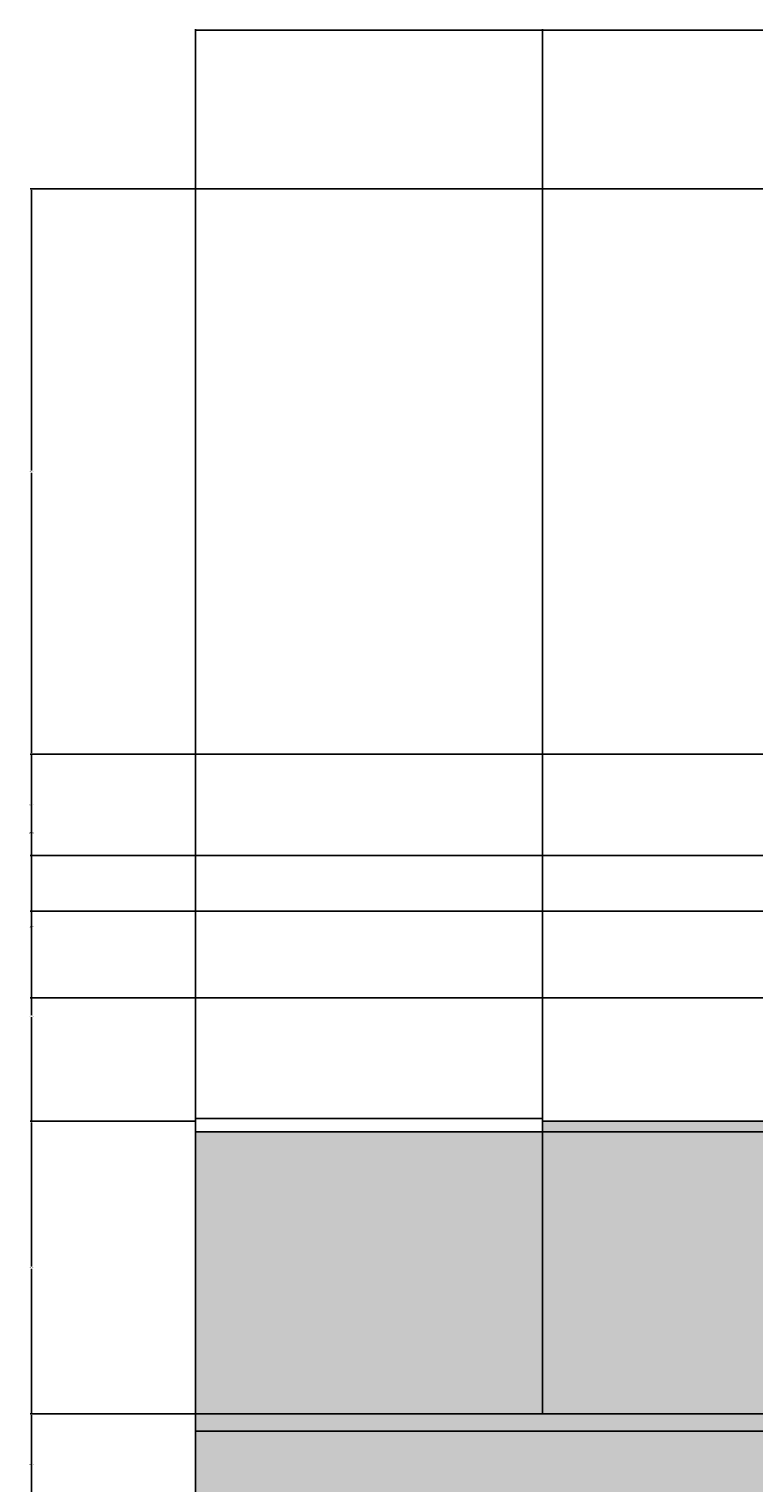
# Model space of a CAD drawing. Units: feet. Extents: x 2926 to 4178, y 965 to 1469.
# Tile 4 of 9: x 2926 to 3040, y 1241 to 1469. Entities that reach past the tile are written whole.
import ezdxf

# ---------------------------------------------------------------- set-up
doc = ezdxf.new("R2010")
doc.units = ezdxf.units.FT
for name, color, linetype, lineweight in [('A-ANNO-DIMS', 2, 'Continuous', 18), ('A-ELEV', 7, 'Continuous', 25), ('A-ELEV-PATT', 9, 'Continuous', 13)]:
    doc.layers.add(name, color=color, linetype=linetype, lineweight=lineweight)
doc.styles.get("Standard").update_dxf_attribs({"font": 'arial.ttf'})
doc.dimstyles.get("Standard").update_dxf_attribs({"dimtxt": 0.18, "dimasz": 0.18, "dimexe": 0.18, "dimexo": 0.0625, "dimgap": 0.09, "dimtad": 0, "dimtih": 1, "dimtoh": 1, "dimdec": 1, "dimzin": 0, "dimdsep": 46, "dimlunit": 3, "dimtxsty": 'Standard', "dimcen": 0.09, "dimadec": 0, "dimazin": 0, "dimtfac": 1, "dimtdec": 1, "dimtofl": 0, "dimtmove": 0, "dimatfit": 3, "dimfxl": 1, "dimtolj": 1, "dimtzin": 0, "dimarcsym": 0})

# ---------------------------------------------------------------- blocks, each defined once
blk = doc.blocks.new('*D10')
at = {"layer": 'A-ANNO-DIMS', "color": 0, "lineweight": -2, "transparency": 16777216}
for p, q in [((2952.4, 1298.4), (2952.4, 1468.62)), ((2952.58, 1468.44), (3195.09, 1468.44)), ((3438.39, 1468.44), (3195.88, 1468.44)), ((3438.57, 1443.71), (3438.57, 1468.62))]:
    blk.add_line(p, q, dxfattribs=at)
at = {"layer": 'A-ANNO-DIMS', "color": 0, "transparency": 16777216}
for points in [[(2952.58, 1468.47), (2952.58, 1468.41), (2952.4, 1468.44)], [(3438.39, 1468.47), (3438.39, 1468.41), (3438.57, 1468.44)]]:
    blk.add_solid(points, dxfattribs=at)
at = {"layer": 'Defpoints', "color": 0, "transparency": 16777216}
for p in [(3438.57, 1468.44), (3438.57, 1443.64), (2952.4, 1298.33)]:
    blk.add_point(p, dxfattribs=at)
at = {"layer": 'A-ANNO-DIMS', "color": 0, "transparency": 16777216, "insert": (3195.49, 1468.44), "char_height": 0.18, "attachment_point": 5}
blk.add_mtext('\\A1;486.2', dxfattribs=at)
blk = doc.blocks.new('*D17')
at = {"layer": 'A-ANNO-DIMS', "color": 0, "lineweight": -2, "transparency": 16777216}
for p, q in [((2952.34, 1252.14), (2926.57, 1252.14)), ((2926.75, 1251.96), (2926.75, 1235.86)), ((2926.75, 1219.4), (2926.75, 1235.5)), ((3198.58, 1219.22), (2926.57, 1219.22))]:
    blk.add_line(p, q, dxfattribs=at)
at = {"layer": 'A-ANNO-DIMS', "color": 0, "transparency": 16777216}
for points in [[(2926.72, 1251.96), (2926.78, 1251.96), (2926.75, 1252.14)], [(2926.72, 1219.4), (2926.78, 1219.4), (2926.75, 1219.22)]]:
    blk.add_solid(points, dxfattribs=at)
at = {"layer": 'Defpoints', "color": 0, "transparency": 16777216}
for p in [(2926.75, 1252.14), (2952.4, 1252.14), (3198.64, 1219.22)]:
    blk.add_point(p, dxfattribs=at)
at = {"layer": 'A-ANNO-DIMS', "color": 0, "transparency": 16777216, "insert": (2926.75, 1235.68), "char_height": 0.18, "attachment_point": 5}
blk.add_mtext('\\A1;32.92', dxfattribs=at)
blk = doc.blocks.new('*D18')
at = {"layer": 'A-ANNO-DIMS', "color": 0, "lineweight": -2, "transparency": 16777216}
for p, q in [((2952.34, 1297.9), (2926.57, 1297.9)), ((2926.75, 1297.72), (2926.75, 1275.2)), ((2926.75, 1252.32), (2926.75, 1274.84)), ((2952.34, 1252.14), (2926.57, 1252.14))]:
    blk.add_line(p, q, dxfattribs=at)
at = {"layer": 'A-ANNO-DIMS', "color": 0, "transparency": 16777216}
for points in [[(2926.72, 1297.72), (2926.78, 1297.72), (2926.75, 1297.9)], [(2926.72, 1252.32), (2926.78, 1252.32), (2926.75, 1252.14)]]:
    blk.add_solid(points, dxfattribs=at)
at = {"layer": 'Defpoints', "color": 0, "transparency": 16777216}
for p in [(2926.75, 1297.9), (2952.4, 1297.9), (2952.4, 1252.14)]:
    blk.add_point(p, dxfattribs=at)
at = {"layer": 'A-ANNO-DIMS', "color": 0, "transparency": 16777216, "insert": (2926.75, 1275.02), "char_height": 0.18, "attachment_point": 5}
blk.add_mtext('\\A1;45.76', dxfattribs=at)
blk = doc.blocks.new('*D19')
at = {"layer": 'A-ANNO-DIMS', "color": 0, "lineweight": -2, "transparency": 16777216}
for p, q in [((3335.85, 1330.74), (2926.57, 1330.74)), ((2926.75, 1330.56), (2926.75, 1314.5)), ((2926.75, 1298.08), (2926.75, 1314.14)), ((2952.34, 1297.9), (2926.57, 1297.9))]:
    blk.add_line(p, q, dxfattribs=at)
at = {"layer": 'A-ANNO-DIMS', "color": 0, "transparency": 16777216}
for points in [[(2926.72, 1330.56), (2926.78, 1330.56), (2926.75, 1330.74)], [(2926.72, 1298.08), (2926.78, 1298.08), (2926.75, 1297.9)]]:
    blk.add_solid(points, dxfattribs=at)
at = {"layer": 'Defpoints', "color": 0, "transparency": 16777216}
for p in [(2926.75, 1330.74), (3335.91, 1330.74), (2952.4, 1297.9)]:
    blk.add_point(p, dxfattribs=at)
at = {"layer": 'A-ANNO-DIMS', "color": 0, "transparency": 16777216, "insert": (2926.75, 1314.32), "char_height": 0.18, "attachment_point": 5}
blk.add_mtext('\\A1;32.85', dxfattribs=at)
blk = doc.blocks.new('*D20')
at = {"layer": 'A-ANNO-DIMS', "color": 0, "lineweight": -2, "transparency": 16777216}
for p, q in [((3042.86, 1355.28), (2926.57, 1355.28)), ((2926.75, 1355.1), (2926.75, 1343.19)), ((2926.75, 1330.92), (2926.75, 1342.83)), ((3335.85, 1330.74), (2926.57, 1330.74))]:
    blk.add_line(p, q, dxfattribs=at)
at = {"layer": 'A-ANNO-DIMS', "color": 0, "transparency": 16777216}
for points in [[(2926.72, 1355.1), (2926.78, 1355.1), (2926.75, 1355.28)], [(2926.72, 1330.92), (2926.78, 1330.92), (2926.75, 1330.74)]]:
    blk.add_solid(points, dxfattribs=at)
at = {"layer": 'Defpoints', "color": 0, "transparency": 16777216}
for p in [(2926.75, 1355.28), (3042.92, 1355.28), (3335.91, 1330.74)]:
    blk.add_point(p, dxfattribs=at)
at = {"layer": 'A-ANNO-DIMS', "color": 0, "transparency": 16777216, "insert": (2926.75, 1343.01), "char_height": 0.18, "attachment_point": 5}
blk.add_mtext('\\A1;24.533', dxfattribs=at)
blk = doc.blocks.new('*D21')
at = {"layer": 'A-ANNO-DIMS', "color": 0, "lineweight": -2, "transparency": 16777216}
for p, q in [((3153.63, 1443.64), (2926.57, 1443.64)), ((2926.75, 1443.46), (2926.75, 1399.64)), ((2926.75, 1355.46), (2926.75, 1399.28)), ((3042.86, 1355.28), (2926.57, 1355.28))]:
    blk.add_line(p, q, dxfattribs=at)
at = {"layer": 'A-ANNO-DIMS', "color": 0, "transparency": 16777216}
for points in [[(2926.72, 1443.46), (2926.78, 1443.46), (2926.75, 1443.64)], [(2926.72, 1355.46), (2926.78, 1355.46), (2926.75, 1355.28)]]:
    blk.add_solid(points, dxfattribs=at)
at = {"layer": 'Defpoints', "color": 0, "transparency": 16777216}
for p in [(2926.75, 1443.64), (3153.7, 1443.64), (3042.92, 1355.28)]:
    blk.add_point(p, dxfattribs=at)
at = {"layer": 'A-ANNO-DIMS', "color": 0, "transparency": 16777216, "insert": (2926.75, 1399.46), "char_height": 0.18, "attachment_point": 5}
blk.add_mtext('\\A1;88.37', dxfattribs=at)
blk = doc.blocks.new('*D22')
at = {"layer": 'A-ANNO-DIMS', "color": 0, "lineweight": -2, "transparency": 16777216}
for p, q in [((2952.4, 1056.38), (2952.4, 1468.62)), ((2952.58, 1468.44), (3009.97, 1468.44)), ((3068.13, 1468.44), (3010.74, 1468.44)), ((3068.31, 1050.05), (3068.31, 1468.62))]:
    blk.add_line(p, q, dxfattribs=at)
at = {"layer": 'A-ANNO-DIMS', "color": 0, "transparency": 16777216}
for points in [[(2952.58, 1468.47), (2952.58, 1468.41), (2952.4, 1468.44)], [(3068.13, 1468.47), (3068.13, 1468.41), (3068.31, 1468.44)]]:
    blk.add_solid(points, dxfattribs=at)
at = {"layer": 'Defpoints', "color": 0, "transparency": 16777216}
for p in [(3068.31, 1468.44), (2952.4, 1056.32), (3068.31, 1049.98)]:
    blk.add_point(p, dxfattribs=at)
at = {"layer": 'A-ANNO-DIMS', "color": 0, "transparency": 16777216, "insert": (3010.36, 1468.44), "char_height": 0.18, "attachment_point": 5}
blk.add_mtext('\\A1;115.9', dxfattribs=at)
blk = doc.blocks.new('*D29')
at = {"layer": 'A-ANNO-DIMS', "color": 0, "lineweight": -2, "transparency": 16777216}
for p, q in [((2952.4, 1298.4), (2952.4, 1468.62)), ((2952.58, 1468.44), (2997.27, 1468.44)), ((3042.74, 1468.44), (2998.05, 1468.44)), ((3042.92, 1355.34), (3042.92, 1468.62))]:
    blk.add_line(p, q, dxfattribs=at)
at = {"layer": 'A-ANNO-DIMS', "color": 0, "transparency": 16777216}
for points in [[(2952.58, 1468.47), (2952.58, 1468.41), (2952.4, 1468.44)], [(3042.74, 1468.47), (3042.74, 1468.41), (3042.92, 1468.44)]]:
    blk.add_solid(points, dxfattribs=at)
at = {"layer": 'Defpoints', "color": 0, "transparency": 16777216}
for p in [(3042.92, 1468.44), (3042.92, 1355.28), (2952.4, 1298.33)]:
    blk.add_point(p, dxfattribs=at)
at = {"layer": 'A-ANNO-DIMS', "color": 0, "transparency": 16777216, "insert": (2997.66, 1468.44), "char_height": 0.18, "attachment_point": 5}
blk.add_mtext('\\A1;90.52', dxfattribs=at)
blk = doc.blocks.new('*D41')
at = {"layer": 'A-ANNO-DIMS', "color": 0, "lineweight": -2, "transparency": 16777216}
for p, q in [((3042.86, 1355.28), (2926.57, 1355.28)), ((2926.75, 1355.1), (2926.75, 1347.55)), ((2926.75, 1339.64), (2926.75, 1347.19)), ((3042.86, 1339.46), (2926.57, 1339.46))]:
    blk.add_line(p, q, dxfattribs=at)
at = {"layer": 'A-ANNO-DIMS', "color": 0, "transparency": 16777216}
for points in [[(2926.72, 1355.1), (2926.78, 1355.1), (2926.75, 1355.28)], [(2926.72, 1339.64), (2926.78, 1339.64), (2926.75, 1339.46)]]:
    blk.add_solid(points, dxfattribs=at)
at = {"layer": 'Defpoints', "color": 0, "transparency": 16777216}
for p in [(2926.75, 1355.28), (3042.92, 1355.28), (3042.92, 1339.46)]:
    blk.add_point(p, dxfattribs=at)
at = {"layer": 'A-ANNO-DIMS', "color": 0, "transparency": 16777216, "insert": (2926.75, 1347.37), "char_height": 0.18, "attachment_point": 5}
blk.add_mtext('\\A1;15.814', dxfattribs=at)
blk = doc.blocks.new('*D42')
at = {"layer": 'A-ANNO-DIMS', "color": 0, "lineweight": -2, "transparency": 16777216}
for p, q in [((3042.86, 1339.46), (2926.57, 1339.46)), ((2926.75, 1339.28), (2926.75, 1328.51)), ((2926.75, 1317.36), (2926.75, 1328.14)), ((3070.62, 1317.18), (2926.57, 1317.18))]:
    blk.add_line(p, q, dxfattribs=at)
at = {"layer": 'A-ANNO-DIMS', "color": 0, "transparency": 16777216}
for points in [[(2926.72, 1339.28), (2926.78, 1339.28), (2926.75, 1339.46)], [(2926.72, 1317.36), (2926.78, 1317.36), (2926.75, 1317.18)]]:
    blk.add_solid(points, dxfattribs=at)
at = {"layer": 'Defpoints', "color": 0, "transparency": 16777216}
for p in [(2926.75, 1339.46), (3042.92, 1339.46), (3070.68, 1317.18)]:
    blk.add_point(p, dxfattribs=at)
at = {"layer": 'A-ANNO-DIMS', "color": 0, "transparency": 16777216, "insert": (2926.75, 1328.32), "char_height": 0.18, "attachment_point": 5}
blk.add_mtext('\\A1;22.28', dxfattribs=at)
blk = doc.blocks.new('*D45')
at = {"layer": 'A-ANNO-DIMS', "color": 0, "lineweight": -2, "transparency": 16777216}
for p, q in [((2952.4, 1298.4), (2952.4, 1468.62)), ((2952.58, 1468.44), (2979.13, 1468.44)), ((3006.47, 1468.44), (2979.92, 1468.44)), ((3006.65, 1298.4), (3006.65, 1468.62))]:
    blk.add_line(p, q, dxfattribs=at)
at = {"layer": 'A-ANNO-DIMS', "color": 0, "transparency": 16777216}
for points in [[(2952.58, 1468.47), (2952.58, 1468.41), (2952.4, 1468.44)], [(3006.47, 1468.47), (3006.47, 1468.41), (3006.65, 1468.44)]]:
    blk.add_solid(points, dxfattribs=at)
at = {"layer": 'Defpoints', "color": 0, "transparency": 16777216}
for p in [(3006.65, 1468.44), (2952.4, 1298.33), (3006.65, 1298.33)]:
    blk.add_point(p, dxfattribs=at)
at = {"layer": 'A-ANNO-DIMS', "color": 0, "transparency": 16777216, "insert": (2979.53, 1468.44), "char_height": 0.18, "attachment_point": 5}
blk.add_mtext('\\A1;54.25', dxfattribs=at)
blk = doc.blocks.new('*D46')
at = {"layer": 'A-ANNO-DIMS', "color": 0, "lineweight": -2, "transparency": 16777216}
for p, q in [((3006.65, 1252.2), (3006.65, 1468.62)), ((3006.83, 1468.44), (3038.27, 1468.44)), ((3070.5, 1468.44), (3039.06, 1468.44)), ((3070.68, 1317.25), (3070.68, 1468.62))]:
    blk.add_line(p, q, dxfattribs=at)
at = {"layer": 'A-ANNO-DIMS', "color": 0, "transparency": 16777216}
for points in [[(3006.83, 1468.47), (3006.83, 1468.41), (3006.65, 1468.44)], [(3070.5, 1468.47), (3070.5, 1468.41), (3070.68, 1468.44)]]:
    blk.add_solid(points, dxfattribs=at)
at = {"layer": 'Defpoints', "color": 0, "transparency": 16777216}
for p in [(3070.68, 1468.44), (3070.68, 1317.18), (3006.65, 1252.14)]:
    blk.add_point(p, dxfattribs=at)
at = {"layer": 'A-ANNO-DIMS', "color": 0, "transparency": 16777216, "insert": (3038.66, 1468.44), "char_height": 0.18, "attachment_point": 5}
blk.add_mtext('\\A1;64.03', dxfattribs=at)
blk = doc.blocks.new('*D61')
at = {"layer": 'A-ANNO-DIMS', "color": 0, "lineweight": -2, "transparency": 16777216}
for p, q in [((2952.34, 1252.14), (2926.57, 1252.14)), ((2926.75, 1251.96), (2926.75, 1244.41)), ((2926.75, 1236.5), (2926.75, 1244.05)), ((2952.34, 1236.32), (2926.57, 1236.32))]:
    blk.add_line(p, q, dxfattribs=at)
at = {"layer": 'A-ANNO-DIMS', "color": 0, "transparency": 16777216}
for points in [[(2926.72, 1251.96), (2926.78, 1251.96), (2926.75, 1252.14)], [(2926.72, 1236.5), (2926.78, 1236.5), (2926.75, 1236.32)]]:
    blk.add_solid(points, dxfattribs=at)
at = {"layer": 'Defpoints', "color": 0, "transparency": 16777216}
for p in [(2926.75, 1252.14), (2952.4, 1252.14), (2952.4, 1236.32)]:
    blk.add_point(p, dxfattribs=at)
at = {"layer": 'A-ANNO-DIMS', "color": 0, "transparency": 16777216, "insert": (2926.75, 1244.23), "char_height": 0.18, "attachment_point": 5}
blk.add_mtext('\\A1;15.814', dxfattribs=at)

msp = doc.modelspace()

# ---------------------------------------------------------------- hatches: boundary and pattern name
at = {"layer": 'A-ELEV-PATT'}
h = msp.add_hatch(color=256, dxfattribs=at)
h.dxf.hatch_style = 1
h.paths.add_polyline_path([(2968.9852, 1110.3246), (2958.1139, 1110.3246), (2958.1139, 1060.462), (2968.9852, 1060.462)])
h.paths.add_polyline_path([(3174.217, 1126.1389), (2952.4018, 1126.1389), (2952.4018, 1110.3246), (3174.217, 1110.3246), (3273.5987, 1110.3246), (3273.5987, 1116.3246), (3174.217, 1116.3246)], flags=17)
h.paths.add_polyline_path([(3289.413, 1252.1389), (2952.4018, 1252.1389), (2952.4018, 1236.3246), (3273.5987, 1236.3246), (3273.5987, 1110.3246), (3289.413, 1110.3246)])
h.paths.add_polyline_path([(3221.3497, 1355.2778), (3042.9199, 1355.2778), (3042.9199, 1339.4635), (3221.3497, 1339.4635)])
h.paths.add_polyline_path([(3379.9311, 1355.2778), (3262.1646, 1355.2778), (3262.1646, 1339.4635), (3364.1168, 1339.4635), (3364.1168, 990.3246), (3379.9311, 990.3246)])
h.paths.add_polyline_path([(3364.1168, 1330.7444), (3335.9143, 1330.7444), (3335.9143, 1023.8561), (3364.1168, 1023.8561), (3364.1168, 1027.6935), (3339.7517, 1027.6935), (3339.7517, 1326.907), (3364.1168, 1326.907)], flags=17)
h.paths.add_polyline_path([(3438.5707, 1443.6445), (3153.6951, 1443.6445), (3153.6951, 1427.8302), (3438.5707, 1427.8302)])
h.paths.add_polyline_path([(3174.217, 1427.8302), (3153.6951, 1427.8302), (3174.217, 1356.4366)])
h.paths.add_polyline_path([(3174.217, 1339.4635), (3042.9199, 1339.4635), (3070.6809, 1317.1829), (3174.217, 1317.1829)])
h.paths.add_polyline_path([(3244.819, 1219.2195), (3198.6415, 1219.2195), (3198.6415, 1133.2879), (3244.819, 1133.2879)], flags=17)
h = msp.add_hatch(color=256, dxfattribs=at)
h.dxf.hatch_style = 1
h.paths.add_polyline_path([(3006.649, 1296.2176), (2952.4018, 1296.2176), (2952.4018, 1252.1389), (3006.649, 1252.1389)])
h.paths.add_polyline_path([(3084.0314, 1226.8042), (3008.2802, 1226.8042), (3008.2802, 1171.8963), (3084.0314, 1171.8963)])
h.paths.add_polyline_path([(3004.9276, 1228.4641), (2995.6704, 1228.4641), (2995.6704, 1171.8963), (3004.9276, 1171.8963)])
h.paths.add_polyline_path([(3174.217, 1236.3246), (3084.0314, 1236.3246), (3084.0314, 1171.8963), (3124.7575, 1171.8963), (3124.7575, 1207.1083), (3154.7729, 1207.1083), (3154.7729, 1171.8963), (3174.217, 1171.8963)])
h.paths.add_polyline_path([(3273.5987, 1236.3246), (3174.217, 1236.3246), (3174.217, 1171.8963), (3174.217, 1126.1389), (3174.217, 1116.3246), (3273.5987, 1116.3246)], flags=16)
h.paths.add_polyline_path([(3198.6415, 1219.2195), (3244.819, 1219.2195), (3244.819, 1133.2879), (3198.6415, 1133.2879)], flags=0)
h.paths.add_polyline_path([(3432.4018, 1427.8302), (3174.217, 1427.8302), (3174.217, 1356.4366), (3174.5501, 1355.2778), (3221.3497, 1355.2778), (3221.3497, 1364.3965), (3232.8063, 1364.3965), (3232.8063, 1355.2778), (3236.4098, 1355.2778), (3236.4098, 1364.3965), (3247.8663, 1364.3965), (3247.8663, 1355.2778), (3250.7081, 1355.2778), (3250.7081, 1364.3965), (3262.1646, 1364.3965), (3262.1646, 1355.2778), (3379.9311, 1355.2778), (3379.9311, 990.3246), (3432.4018, 990.3246)])
h.paths.add_polyline_path([(3068.3128, 1092.0439), (3130.6886, 1092.0439), (3130.6886, 1049.9841), (3146.6469, 1049.9841), (3146.6469, 1057.7915), (3145.2184, 1058.2122), (3145.2184, 1060.462), (3168.644, 1060.462), (3174.217, 1058.8204), (3174.217, 1110.3246), (3004.9276, 1110.3246), (3004.9276, 1049.9841), (3068.3128, 1049.9841)])
h.paths.add_polyline_path([(3174.217, 1056.3197), (3152.4954, 1056.3197), (3152.4954, 990.3246), (3174.217, 990.3246)])
h.paths.add_polyline_path([(2974.1234, 1056.3197), (2952.4018, 1056.3197), (2952.4018, 990.3246), (2974.1234, 990.3246)])
h.paths.add_polyline_path([(3004.9276, 1110.3246), (2995.6704, 1110.3246), (2995.6704, 1049.9841), (3004.9276, 1049.9841)])
h = msp.add_hatch(color=256, dxfattribs=at)
h.dxf.hatch_style = 1
h.paths.add_polyline_path([(3174.217, 1297.8963), (3172.3488, 1297.8963), (3006.649, 1297.8963), (3006.649, 1296.2176), (3087.9974, 1296.2176), (3087.9974, 1252.1389), (3089.8656, 1252.1389), (3089.8656, 1296.2176), (3172.3488, 1296.2176), (3172.3488, 1252.1389), (3174.217, 1252.1389)])
h.paths.add_polyline_path([(3102.4583, 1170.2176), (3172.3488, 1170.2176), (3172.3488, 1126.1389), (3174.217, 1126.1389), (3174.217, 1171.8963), (3172.3488, 1171.8963), (2952.4018, 1171.8963), (2952.4018, 1170.2176), (2952.4018, 1126.1389), (2954.27, 1126.1389), (2954.27, 1170.2176), (3100.5901, 1170.2176), (3100.5901, 1126.1389), (3102.4583, 1126.1389)])
h.paths.add_polyline_path([(3130.6886, 1092.0439), (3068.3128, 1092.0439), (3068.3128, 1049.9841), (3130.6886, 1049.9841)])
h.paths.add_polyline_path([(3099.0016, 1090.4638), (3099.0016, 1051.5643), (3069.893, 1051.5643), (3069.893, 1090.4638)], flags=16)
h.paths.add_polyline_path([(3099.9998, 1090.4638), (3129.1085, 1090.4638), (3129.1085, 1051.5643), (3099.9998, 1051.5643)], flags=16)
h.paths.add_polyline_path([(3067.2712, 1049.9841), (3060.102, 1049.9841), (3060.102, 990.3246), (3067.2712, 990.3246)])
h.paths.add_polyline_path([(3339.7517, 1326.907), (3364.1168, 1326.907), (3364.1168, 1330.7444), (3335.9143, 1330.7444), (3335.9143, 1023.8561), (3364.1168, 1023.8561), (3364.1168, 1027.6935), (3339.7517, 1027.6935)])
h.paths.add_polyline_path([(3154.7729, 1207.1083), (3124.7575, 1207.1083), (3124.7575, 1171.8963), (3126.8684, 1171.8963), (3126.8684, 1204.9974), (3152.6619, 1204.9974), (3152.6619, 1171.8963), (3154.7729, 1171.8963)])
h = msp.add_hatch(color=256, dxfattribs=at)
h.dxf.hatch_style = 1
h.paths.add_polyline_path([(3070.6809, 1296.2176), (3006.649, 1296.2176), (3006.649, 1252.1389), (3070.6809, 1252.1389)])
h.paths.add_polyline_path([(3087.9974, 1296.2176), (3070.6809, 1296.2176), (3070.6809, 1252.1389), (3087.9974, 1252.1389)])
h.paths.add_polyline_path([(3172.3488, 1296.2176), (3089.8656, 1296.2176), (3089.8656, 1252.1389), (3172.3488, 1252.1389)])
h.paths.add_polyline_path([(3152.6619, 1170.2176), (3126.8684, 1170.2176), (3126.8684, 1128.2498), (3152.6619, 1128.2498)], flags=17)
h.paths.add_polyline_path([(3152.6619, 1204.9974), (3126.8684, 1204.9974), (3126.8684, 1171.8963), (3152.6619, 1171.8963)])
h.paths.add_polyline_path([(3172.3488, 1170.2176), (3154.7729, 1170.2176), (3154.7729, 1126.1389), (3172.3488, 1126.1389)])
h.paths.add_polyline_path([(3154.7729, 1170.2176), (3152.6619, 1170.2176), (3152.6619, 1128.2498), (3126.8684, 1128.2498), (3126.8684, 1170.2176), (3124.7575, 1170.2176), (3124.7575, 1126.1389), (3154.7729, 1126.1389)])
h.paths.add_polyline_path([(3124.7575, 1170.2176), (3102.4583, 1170.2176), (3102.4583, 1126.1389), (3124.7575, 1126.1389)])
h.paths.add_polyline_path([(3100.5901, 1170.2176), (3084.0314, 1170.2176), (3084.0314, 1126.1389), (3100.5901, 1126.1389)])
h.paths.add_polyline_path([(3084.0314, 1170.2176), (3008.2802, 1170.2176), (3008.2802, 1126.1389), (3084.0314, 1126.1389)])
h.paths.add_polyline_path([(2995.6704, 1170.2176), (2971.1978, 1170.2176), (2971.1978, 1126.1389), (2995.6704, 1126.1389)])
h.paths.add_polyline_path([(3004.9276, 1170.2176), (2995.6704, 1170.2176), (2995.6704, 1126.1389), (3004.9276, 1126.1389)])
h.paths.add_polyline_path([(3364.1168, 1326.907), (3339.7517, 1326.907), (3339.7517, 1027.6935), (3364.1168, 1027.6935)])
h.paths.add_polyline_path([(3099.0016, 1090.4638), (3069.893, 1090.4638), (3069.893, 1051.5643), (3099.0016, 1051.5643)])
h.paths.add_polyline_path([(3129.1085, 1090.4638), (3099.9998, 1090.4638), (3099.9998, 1051.5643), (3129.1085, 1051.5643)])
h.paths.add_polyline_path([(2968.9852, 1170.2176), (2958.1139, 1170.2176), (2958.1139, 1126.1389), (2968.9852, 1126.1389)])
h.paths.add_polyline_path([(2958.1139, 1170.2176), (2954.27, 1170.2176), (2954.27, 1126.1389), (2958.1139, 1126.1389)])
h.paths.add_polyline_path([(2971.1978, 1170.2176), (2968.9852, 1170.2176), (2968.9852, 1126.1389), (2971.1978, 1126.1389)])

# ---------------------------------------------------------------- linework, layer by layer
at = {"layer": 'A-ELEV'}
for p, q in [((2952.4018, 1236.3246), (2952.4018, 1298.3338)), ((2952.4018, 1236.3246), (2952.4018, 1298.3338)), ((2952.4018, 1249.4671), (3289.413, 1249.4671))]:
    msp.add_line(p, q, dxfattribs=at)
for points in [[(3006.649, 1296.2176), (2952.4018, 1296.2176), (2952.4018, 1298.3338), (3006.649, 1298.3338)], [(3006.649, 1296.2176), (2952.4018, 1296.2176), (2952.4018, 1298.3338), (3006.649, 1298.3338)], [(2952.4018, 1296.2176), (3006.649, 1296.2176), (3006.649, 1252.1389), (2952.4018, 1252.1389)], [(2952.4018, 1296.2176), (3006.649, 1296.2176), (3006.649, 1252.1389), (2952.4018, 1252.1389)]]:
    msp.add_lwpolyline(points, close=True, dxfattribs=at)
for points in [[(2952.4018, 1297.8963), (2952.4018, 1296.2176), (3174.217, 1296.2176), (3174.217, 1297.8963), (3006.649, 1297.8963)], [(2952.4018, 1297.8963), (2952.4018, 1296.2176), (3174.217, 1296.2176), (3174.217, 1297.8963), (3006.649, 1297.8963)], [(3289.413, 1236.3246), (3289.413, 1252.1389), (2952.4018, 1252.1389), (2952.4018, 1236.3246), (3273.5987, 1236.3246)], [(3289.413, 1236.3246), (3289.413, 1252.1389), (2952.4018, 1252.1389), (2952.4018, 1236.3246), (3273.5987, 1236.3246)]]:
    msp.add_lwpolyline(points, dxfattribs=at)

# ---------------------------------------------------------------- dimensions: what is measured, and where the dimension line sits
at = {"layer": 'A-ANNO-DIMS'}
for base, p1, p2, override, picture, middle in [((3438.5707, 1468.4445), (2952.4018, 1298.3338), (3438.5707, 1443.6445), {"dimdec": 1, "dimlfac": 1, "dimrnd": 0, "dimzin": 0, "dimdsep": 46, "dimlunit": 2}, '*D10', (3195.4862, 1468.4445)), ((3068.3128, 1468.4445), (2952.4018, 1056.3197), (3068.3128, 1049.9841), {"dimdec": 1, "dimlfac": 1, "dimrnd": 0, "dimzin": 0, "dimdsep": 46, "dimlunit": 2}, '*D22', (3010.3573, 1468.4445)), ((3042.9199, 1468.4445), (2952.4018, 1298.3338), (3042.9199, 1355.2778), {"dimdec": 2, "dimlfac": 1, "dimrnd": 0, "dimzin": 0, "dimdsep": 46, "dimlunit": 2}, '*D29', (2997.6609, 1468.4445)), ((3006.649, 1468.4445), (2952.4018, 1298.3338), (3006.649, 1298.3338), {"dimdec": 2, "dimlfac": 1, "dimrnd": 0, "dimzin": 0, "dimdsep": 46, "dimlunit": 2}, '*D45', (2979.5254, 1468.4445)), ((3070.6809, 1468.4445), (3006.649, 1252.1389), (3070.6809, 1317.1829), {"dimdec": 2, "dimlfac": 1, "dimrnd": 0, "dimzin": 0, "dimdsep": 46, "dimlunit": 2}, '*D46', (3038.665, 1468.4445))]:
    dim = msp.add_linear_dim(base=base, p1=p1, p2=p2, dimstyle='Standard', override=override, dxfattribs=at)
    dim.commit()
    dim.dimension.update_dxf_attribs({"geometry": picture, "text_midpoint": middle})
for base, p1, p2, override, picture, middle in [((2926.7498, 1443.6445), (3042.9199, 1355.2778), (3153.6951, 1443.6445), {"dimdec": 2, "dimlfac": 1, "dimrnd": 0, "dimzin": 0, "dimdsep": 46, "dimlunit": 2}, '*D21', (2926.7498, 1399.4612)), ((2926.7498, 1355.2778), (3335.9143, 1330.7444), (3042.9199, 1355.2778), {"dimdec": 3, "dimlfac": 1, "dimrnd": 0, "dimzin": 0, "dimdsep": 46, "dimlunit": 2}, '*D20', (2926.7498, 1343.0111)), ((2926.7498, 1355.2778), (3042.9199, 1339.4635), (3042.9199, 1355.2778), {"dimdec": 3, "dimlfac": 1, "dimrnd": 0, "dimzin": 0, "dimdsep": 46, "dimlunit": 2}, '*D41', (2926.7498, 1347.3707)), ((2926.7498, 1339.4635), (3070.6809, 1317.1829), (3042.9199, 1339.4635), {"dimdec": 2, "dimlfac": 1, "dimrnd": 0, "dimzin": 0, "dimdsep": 46, "dimlunit": 2}, '*D42', (2926.7498, 1328.3232)), ((2926.7498, 1330.7444), (2952.4018, 1297.8963), (3335.9143, 1330.7444), {"dimdec": 2, "dimlfac": 1, "dimrnd": 0, "dimzin": 0, "dimdsep": 46, "dimlunit": 2}, '*D19', (2926.7498, 1314.3203)), ((2926.7498, 1297.8963), (2952.4018, 1252.1389), (2952.4018, 1297.8963), {"dimdec": 2, "dimlfac": 1, "dimrnd": 0, "dimzin": 0, "dimdsep": 46, "dimlunit": 2}, '*D18', (2926.7498, 1275.0176)), ((2926.7498, 1252.1389), (2952.4018, 1236.3246), (2952.4018, 1252.1389), {"dimdec": 3, "dimlfac": 1, "dimrnd": 0, "dimzin": 0, "dimdsep": 46, "dimlunit": 2}, '*D61', (2926.7498, 1244.2317)), ((2926.7498, 1252.1389), (3198.6415, 1219.2195), (2952.4018, 1252.1389), {"dimdec": 2, "dimlfac": 1, "dimrnd": 0, "dimzin": 0, "dimdsep": 46, "dimlunit": 2}, '*D17', (2926.7498, 1235.6792))]:
    dim = msp.add_linear_dim(base=base, p1=p1, p2=p2, angle=90, dimstyle='Standard', override=override, dxfattribs=at)
    dim.commit()
    dim.dimension.update_dxf_attribs({"geometry": picture, "text_midpoint": middle})

doc.saveas('drawing.dxf')
